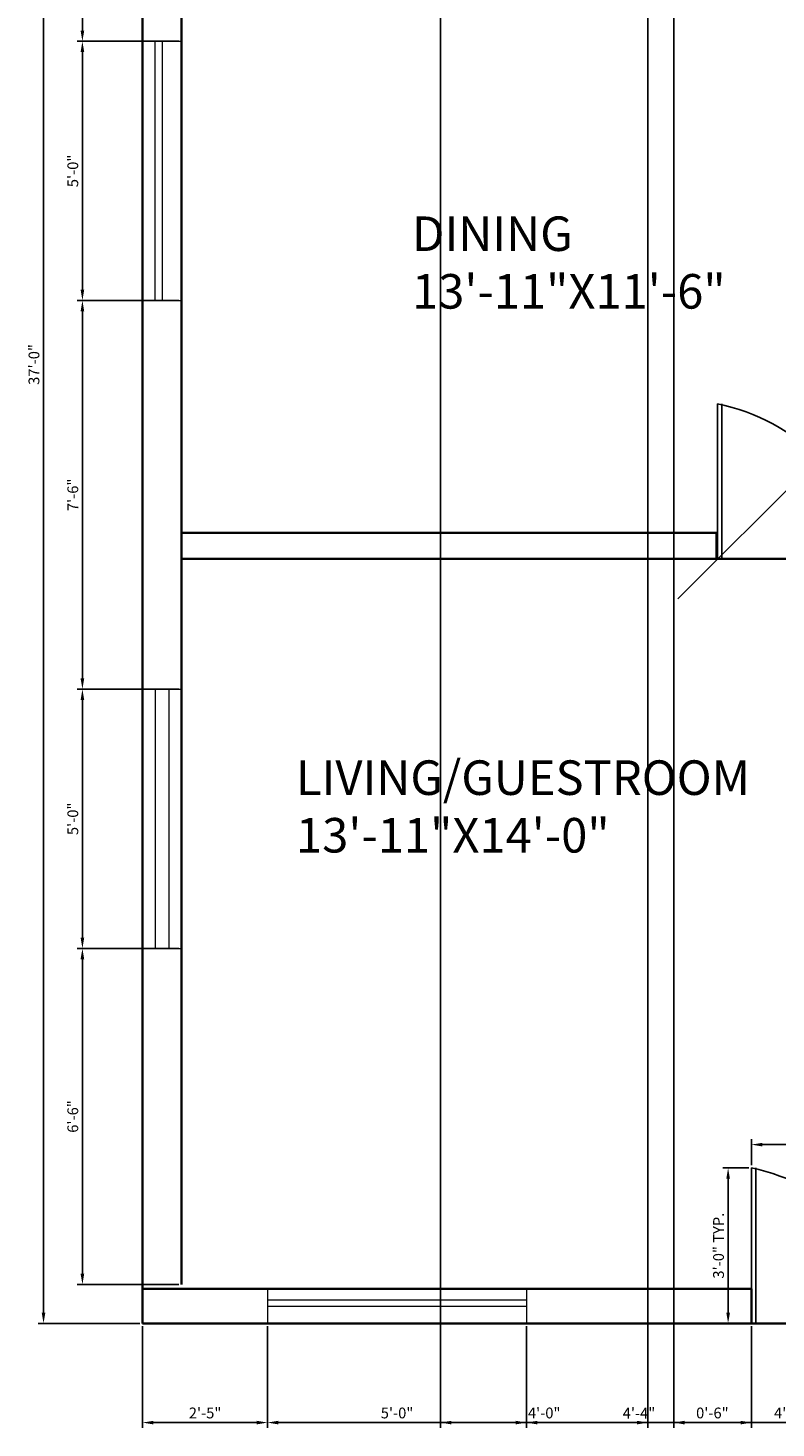
# Model space of a CAD drawing. Units: inches. Extents: x -2945 to -2182, y 3541 to 4172.
# Tile 3 of 5: x -2558 to -2384, y 3541 to 3865. Entities that reach past the tile are written whole.
import ezdxf

# ---------------------------------------------------------------- set-up
doc = ezdxf.new("R2010")
doc.units = ezdxf.units.IN
for name, color, linetype, lineweight in [('A-ANNO-DIMS', 2, 'Continuous', 18), ('A-AREA-IDEN', 7, 'Continuous', 18), ('A-DOOR', 3, 'Continuous', 25), ('A-GLAZ', 4, 'Continuous', 18), ('A-WALL', 7, 'Continuous', 35)]:
    doc.layers.add(name, color=color, linetype=linetype, lineweight=lineweight)
doc.styles.get("Standard").update_dxf_attribs({"font": 'arial.ttf'})
doc.dimstyles.new('ISO-25', dxfattribs={"dimtxt": 2.5, "dimasz": 2.5, "dimexe": 1.25, "dimexo": 0.625, "dimtad": 1, "dimdec": 0, "dimlunit": 3, "dimtxsty": 'Standard', "dimcen": 2.5, "dimadec": 0, "dimazin": 0, "dimtfac": 1, "dimtdec": 0, "dimtmove": 0, "dimatfit": 3, "dimfxl": 1, "dimarcsym": 0})

# ---------------------------------------------------------------- blocks, each defined once
blk = doc.blocks.new('DOOR-SINGLE-36IN')
for p, q in [((0, 0), (0, 36)), ((1, 0), (1, 36))]:
    blk.add_line(p, q)
blk.add_arc((-9.18, -9.18), 46.1, 11.4852, 78.5148)
blk = doc.blocks.new('*D18')
at = {"layer": 'A-ANNO-DIMS', "color": 0, "lineweight": -2, "transparency": 16777216}
for p, q in [((-2390.05, 3602.2), (-2390.05, 3608.23)), ((-2354.05, 3602.2), (-2354.05, 3608.23)), ((-2387.55, 3606.98), (-2356.55, 3606.98)), ((-2354.05, 3606.98), (-2309.84, 3606.98))]:
    blk.add_line(p, q, dxfattribs=at)
at = {"layer": 'A-ANNO-DIMS', "color": 0, "transparency": 16777216}
for points in [[(-2387.55, 3607.39), (-2387.55, 3606.56), (-2390.05, 3606.98)], [(-2356.55, 3607.39), (-2356.55, 3606.56), (-2354.05, 3606.98)]]:
    blk.add_solid(points, dxfattribs=at)
at = {"layer": 'Defpoints', "color": 0, "transparency": 16777216}
for p in [(-2354.05, 3606.98), (-2390.05, 3601.58), (-2354.05, 3601.58)]:
    blk.add_point(p, dxfattribs=at)
at = {"layer": 'A-ANNO-DIMS', "color": 0, "transparency": 16777216, "insert": (-2330.7, 3608.89), "char_height": 2.5, "attachment_point": 5}
blk.add_mtext('SINGLE DOOR 3\'-0" TYP.', dxfattribs=at)
blk = doc.blocks.new('*D19')
at = {"layer": 'A-ANNO-DIMS', "color": 0, "lineweight": -2, "transparency": 16777216}
for p, q in [((-2390.67, 3601.58), (-2396.7, 3601.58)), ((-2395.45, 3568.08), (-2395.45, 3599.08)), ((-2390.67, 3565.58), (-2396.7, 3565.58))]:
    blk.add_line(p, q, dxfattribs=at)
at = {"layer": 'A-ANNO-DIMS', "color": 0, "transparency": 16777216}
for points in [[(-2395.87, 3599.08), (-2395.03, 3599.08), (-2395.45, 3601.58)], [(-2395.87, 3568.08), (-2395.03, 3568.08), (-2395.45, 3565.58)]]:
    blk.add_solid(points, dxfattribs=at)
at = {"layer": 'Defpoints', "color": 0, "transparency": 16777216}
for p in [(-2395.45, 3601.58), (-2390.05, 3601.58), (-2390.05, 3565.58)]:
    blk.add_point(p, dxfattribs=at)
at = {"layer": 'A-ANNO-DIMS', "color": 0, "transparency": 16777216, "insert": (-2397.35, 3583.58), "char_height": 2.5, "attachment_point": 5, "rotation": 90}
blk.add_mtext('3\'-0" TYP.', dxfattribs=at)
blk = doc.blocks.new('*D21')
at = {"layer": 'A-ANNO-DIMS', "color": 0, "lineweight": -2, "transparency": 16777216}
for p, q in [((-2531.67, 4009.58), (-2555.25, 4009.58)), ((-2554, 3568.08), (-2554, 4007.08)), ((-2531.67, 3565.58), (-2555.25, 3565.58))]:
    blk.add_line(p, q, dxfattribs=at)
at = {"layer": 'A-ANNO-DIMS', "color": 0, "transparency": 16777216}
for points in [[(-2554.42, 4007.08), (-2553.58, 4007.08), (-2554, 4009.58)], [(-2554.42, 3568.08), (-2553.58, 3568.08), (-2554, 3565.58)]]:
    blk.add_solid(points, dxfattribs=at)
at = {"layer": 'Defpoints', "color": 0, "transparency": 16777216}
for p in [(-2554, 4009.58), (-2531.05, 4009.58), (-2531.05, 3565.58)]:
    blk.add_point(p, dxfattribs=at)
at = {"layer": 'A-ANNO-DIMS', "color": 0, "transparency": 16777216, "insert": (-2555.9, 3787.58), "char_height": 2.5, "attachment_point": 5, "rotation": 90}
blk.add_mtext('37\'-0"', dxfattribs=at)
blk = doc.blocks.new('*D22')
at = {"layer": 'A-ANNO-DIMS', "color": 0, "lineweight": -2, "transparency": 16777216}
for p, q in [((-2531.05, 3564.95), (-2531.05, 3541.38)), ((-2502.13, 3564.95), (-2502.13, 3541.38)), ((-2528.55, 3542.63), (-2504.63, 3542.63))]:
    blk.add_line(p, q, dxfattribs=at)
at = {"layer": 'A-ANNO-DIMS', "color": 0, "transparency": 16777216}
for points in [[(-2528.55, 3543.04), (-2528.55, 3542.21), (-2531.05, 3542.63)], [(-2504.63, 3543.04), (-2504.63, 3542.21), (-2502.13, 3542.63)]]:
    blk.add_solid(points, dxfattribs=at)
at = {"layer": 'Defpoints', "color": 0, "transparency": 16777216}
for p in [(-2531.05, 3565.58), (-2502.13, 3565.58), (-2502.13, 3542.63)]:
    blk.add_point(p, dxfattribs=at)
at = {"layer": 'A-ANNO-DIMS', "color": 0, "transparency": 16777216, "insert": (-2516.59, 3544.53), "char_height": 2.5, "attachment_point": 5}
blk.add_mtext('2\'-5"', dxfattribs=at)
blk = doc.blocks.new('*D23')
at = {"layer": 'A-ANNO-DIMS', "color": 0, "lineweight": -2, "transparency": 16777216}
for p, q in [((-2502.13, 3564.95), (-2502.13, 3541.38)), ((-2442.13, 3564.95), (-2442.13, 3541.38)), ((-2499.63, 3542.63), (-2444.63, 3542.63))]:
    blk.add_line(p, q, dxfattribs=at)
at = {"layer": 'A-ANNO-DIMS', "color": 0, "transparency": 16777216}
for points in [[(-2499.63, 3543.04), (-2499.63, 3542.21), (-2502.13, 3542.63)], [(-2444.63, 3543.04), (-2444.63, 3542.21), (-2442.13, 3542.63)]]:
    blk.add_solid(points, dxfattribs=at)
at = {"layer": 'Defpoints', "color": 0, "transparency": 16777216}
for p in [(-2502.13, 3565.58), (-2442.13, 3565.58), (-2442.13, 3542.63)]:
    blk.add_point(p, dxfattribs=at)
at = {"layer": 'A-ANNO-DIMS', "color": 0, "transparency": 16777216, "insert": (-2472.13, 3544.53), "char_height": 2.5, "attachment_point": 5}
blk.add_mtext('5\'-0"', dxfattribs=at)
blk = doc.blocks.new('*D24')
at = {"layer": 'A-ANNO-DIMS', "color": 0, "lineweight": -2, "transparency": 16777216}
for p, q in [((-2442.13, 3564.95), (-2442.13, 3541.38)), ((-2390.05, 3564.95), (-2390.05, 3541.38)), ((-2439.63, 3542.63), (-2392.55, 3542.63))]:
    blk.add_line(p, q, dxfattribs=at)
at = {"layer": 'A-ANNO-DIMS', "color": 0, "transparency": 16777216}
for points in [[(-2439.63, 3543.04), (-2439.63, 3542.21), (-2442.13, 3542.63)], [(-2392.55, 3543.04), (-2392.55, 3542.21), (-2390.05, 3542.63)]]:
    blk.add_solid(points, dxfattribs=at)
at = {"layer": 'Defpoints', "color": 0, "transparency": 16777216}
for p in [(-2442.13, 3565.58), (-2390.05, 3565.58), (-2390.05, 3542.63)]:
    blk.add_point(p, dxfattribs=at)
at = {"layer": 'A-ANNO-DIMS', "color": 0, "transparency": 16777216, "insert": (-2416.09, 3544.5), "char_height": 2.5, "attachment_point": 5}
blk.add_mtext('4\'-4"', dxfattribs=at)
blk = doc.blocks.new('*D25')
at = {"layer": 'A-ANNO-DIMS', "color": 0, "lineweight": -2, "transparency": 16777216}
for p, q in [((-2522.67, 3652.4), (-2546.25, 3652.4)), ((-2545, 3577.08), (-2545, 3649.9)), ((-2522.67, 3574.58), (-2546.25, 3574.58))]:
    blk.add_line(p, q, dxfattribs=at)
at = {"layer": 'A-ANNO-DIMS', "color": 0, "transparency": 16777216}
for points in [[(-2545.42, 3649.9), (-2544.58, 3649.9), (-2545, 3652.4)], [(-2545.42, 3577.08), (-2544.58, 3577.08), (-2545, 3574.58)]]:
    blk.add_solid(points, dxfattribs=at)
at = {"layer": 'Defpoints', "color": 0, "transparency": 16777216}
for p in [(-2545, 3652.4), (-2522.05, 3652.4), (-2522.05, 3574.58)]:
    blk.add_point(p, dxfattribs=at)
at = {"layer": 'A-ANNO-DIMS', "color": 0, "transparency": 16777216, "insert": (-2546.9, 3613.49), "char_height": 2.5, "attachment_point": 5, "rotation": 90}
blk.add_mtext('6\'-6"', dxfattribs=at)
blk = doc.blocks.new('*D26')
at = {"layer": 'A-ANNO-DIMS', "color": 0, "lineweight": -2, "transparency": 16777216}
for p, q in [((-2522.67, 3712.4), (-2546.25, 3712.4)), ((-2545, 3654.9), (-2545, 3709.9)), ((-2522.67, 3652.4), (-2546.25, 3652.4))]:
    blk.add_line(p, q, dxfattribs=at)
at = {"layer": 'A-ANNO-DIMS', "color": 0, "transparency": 16777216}
for points in [[(-2545.42, 3709.9), (-2544.58, 3709.9), (-2545, 3712.4)], [(-2545.42, 3654.9), (-2544.58, 3654.9), (-2545, 3652.4)]]:
    blk.add_solid(points, dxfattribs=at)
at = {"layer": 'Defpoints', "color": 0, "transparency": 16777216}
for p in [(-2545, 3712.4), (-2522.05, 3712.4), (-2522.05, 3652.4)]:
    blk.add_point(p, dxfattribs=at)
at = {"layer": 'A-ANNO-DIMS', "color": 0, "transparency": 16777216, "insert": (-2546.9, 3682.4), "char_height": 2.5, "attachment_point": 5, "rotation": 90}
blk.add_mtext('5\'-0"', dxfattribs=at)
blk = doc.blocks.new('*D27')
at = {"layer": 'A-ANNO-DIMS', "color": 0, "lineweight": -2, "transparency": 16777216}
for p, q in [((-2522.67, 3802.39), (-2546.25, 3802.39)), ((-2545, 3714.9), (-2545, 3799.89)), ((-2522.67, 3712.4), (-2546.25, 3712.4))]:
    blk.add_line(p, q, dxfattribs=at)
at = {"layer": 'A-ANNO-DIMS', "color": 0, "transparency": 16777216}
for points in [[(-2545.42, 3799.89), (-2544.58, 3799.89), (-2545, 3802.39)], [(-2545.42, 3714.9), (-2544.58, 3714.9), (-2545, 3712.4)]]:
    blk.add_solid(points, dxfattribs=at)
at = {"layer": 'Defpoints', "color": 0, "transparency": 16777216}
for p in [(-2545, 3802.39), (-2522.05, 3802.39), (-2522.05, 3712.4)]:
    blk.add_point(p, dxfattribs=at)
at = {"layer": 'A-ANNO-DIMS', "color": 0, "transparency": 16777216, "insert": (-2546.9, 3757.4), "char_height": 2.5, "attachment_point": 5, "rotation": 90}
blk.add_mtext('7\'-6"', dxfattribs=at)
blk = doc.blocks.new('*D28')
at = {"layer": 'A-ANNO-DIMS', "color": 0, "lineweight": -2, "transparency": 16777216}
for p, q in [((-2522.67, 3862.39), (-2546.25, 3862.39)), ((-2545, 3804.89), (-2545, 3859.89)), ((-2522.67, 3802.39), (-2546.25, 3802.39))]:
    blk.add_line(p, q, dxfattribs=at)
at = {"layer": 'A-ANNO-DIMS', "color": 0, "transparency": 16777216}
for points in [[(-2545.42, 3859.89), (-2544.58, 3859.89), (-2545, 3862.39)], [(-2545.42, 3804.89), (-2544.58, 3804.89), (-2545, 3802.39)]]:
    blk.add_solid(points, dxfattribs=at)
at = {"layer": 'Defpoints', "color": 0, "transparency": 16777216}
for p in [(-2545, 3862.39), (-2522.05, 3862.39), (-2522.05, 3802.39)]:
    blk.add_point(p, dxfattribs=at)
at = {"layer": 'A-ANNO-DIMS', "color": 0, "transparency": 16777216, "insert": (-2546.9, 3832.39), "char_height": 2.5, "attachment_point": 5, "rotation": 90}
blk.add_mtext('5\'-0"', dxfattribs=at)
blk = doc.blocks.new('*D29')
at = {"layer": 'A-ANNO-DIMS', "color": 0, "lineweight": -2, "transparency": 16777216}
for p, q in [((-2522.67, 3935.75), (-2546.25, 3935.75)), ((-2545, 3864.89), (-2545, 3933.25)), ((-2522.67, 3862.39), (-2546.25, 3862.39))]:
    blk.add_line(p, q, dxfattribs=at)
at = {"layer": 'A-ANNO-DIMS', "color": 0, "transparency": 16777216}
for points in [[(-2545.42, 3933.25), (-2544.58, 3933.25), (-2545, 3935.75)], [(-2545.42, 3864.89), (-2544.58, 3864.89), (-2545, 3862.39)]]:
    blk.add_solid(points, dxfattribs=at)
at = {"layer": 'Defpoints', "color": 0, "transparency": 16777216}
for p in [(-2545, 3935.75), (-2522.05, 3935.75), (-2522.05, 3862.39)]:
    blk.add_point(p, dxfattribs=at)
at = {"layer": 'A-ANNO-DIMS', "color": 0, "transparency": 16777216, "insert": (-2546.92, 3899.07), "char_height": 2.5, "attachment_point": 5, "rotation": 90}
blk.add_mtext('6\'-1 1/2"', dxfattribs=at)
blk = doc.blocks.new('*D41')
at = {"layer": 'A-ANNO-DIMS', "color": 0, "lineweight": -2, "transparency": 16777216}
for p, q in [((-2408.05, 3920.95), (-2408.05, 3541.38)), ((-2354.05, 3920.95), (-2354.05, 3541.38)), ((-2405.55, 3542.63), (-2356.55, 3542.63))]:
    blk.add_line(p, q, dxfattribs=at)
at = {"layer": 'A-ANNO-DIMS', "color": 0, "transparency": 16777216}
for points in [[(-2405.55, 3543.04), (-2405.55, 3542.21), (-2408.05, 3542.63)], [(-2356.55, 3543.04), (-2356.55, 3542.21), (-2354.05, 3542.63)]]:
    blk.add_solid(points, dxfattribs=at)
at = {"layer": 'Defpoints', "color": 0, "transparency": 16777216}
for p in [(-2408.05, 3921.58), (-2354.05, 3921.58), (-2354.05, 3542.63)]:
    blk.add_point(p, dxfattribs=at)
at = {"layer": 'A-ANNO-DIMS', "color": 0, "transparency": 16777216, "insert": (-2381.05, 3544.53), "char_height": 2.5, "attachment_point": 5}
blk.add_mtext('4\'-6"', dxfattribs=at)
blk = doc.blocks.new('*D45')
at = {"layer": 'A-ANNO-DIMS', "color": 0, "lineweight": -2, "transparency": 16777216}
for p, q in [((-2414.05, 3885.95), (-2414.05, 3541.38)), ((-2408.05, 3885.95), (-2408.05, 3541.38)), ((-2416.55, 3542.63), (-2419.05, 3542.63)), ((-2414.05, 3542.63), (-2408.05, 3542.63)), ((-2405.55, 3542.63), (-2395.15, 3542.63))]:
    blk.add_line(p, q, dxfattribs=at)
at = {"layer": 'A-ANNO-DIMS', "color": 0, "transparency": 16777216}
for points in [[(-2416.55, 3543.04), (-2416.55, 3542.21), (-2414.05, 3542.63)], [(-2405.55, 3543.04), (-2405.55, 3542.21), (-2408.05, 3542.63)]]:
    blk.add_solid(points, dxfattribs=at)
at = {"layer": 'Defpoints', "color": 0, "transparency": 16777216}
for p in [(-2414.05, 3886.58), (-2408.05, 3886.58), (-2408.05, 3542.63)]:
    blk.add_point(p, dxfattribs=at)
at = {"layer": 'A-ANNO-DIMS', "color": 0, "transparency": 16777216, "insert": (-2399.1, 3544.53), "char_height": 2.5, "attachment_point": 5}
blk.add_mtext('0\'-6"', dxfattribs=at)
blk = doc.blocks.new('*D47')
at = {"layer": 'A-ANNO-DIMS', "color": 0, "lineweight": -2, "transparency": 16777216}
for p, q in [((-2462.05, 3885.95), (-2462.05, 3541.38)), ((-2414.05, 3885.95), (-2414.05, 3541.38)), ((-2459.55, 3542.63), (-2416.55, 3542.63))]:
    blk.add_line(p, q, dxfattribs=at)
at = {"layer": 'A-ANNO-DIMS', "color": 0, "transparency": 16777216}
for points in [[(-2459.55, 3543.04), (-2459.55, 3542.21), (-2462.05, 3542.63)], [(-2416.55, 3543.04), (-2416.55, 3542.21), (-2414.05, 3542.63)]]:
    blk.add_solid(points, dxfattribs=at)
at = {"layer": 'Defpoints', "color": 0, "transparency": 16777216}
for p in [(-2462.05, 3886.58), (-2414.05, 3886.58), (-2414.05, 3542.63)]:
    blk.add_point(p, dxfattribs=at)
at = {"layer": 'A-ANNO-DIMS', "color": 0, "transparency": 16777216, "insert": (-2438.05, 3544.53), "char_height": 2.5, "attachment_point": 5}
blk.add_mtext('4\'-0"', dxfattribs=at)
blk = doc.blocks.new('*D77')
at = {"layer": 'A-ANNO-DIMS', "color": 0, "lineweight": -2, "transparency": 16777216}
for p, q in [((-2350.58, 3789.78), (-2372.69, 3767.66)), ((-2407.06, 3733.29), (-2374.46, 3765.89))]:
    blk.add_line(p, q, dxfattribs=at)
at = {"layer": 'A-ANNO-DIMS', "color": 0, "transparency": 16777216}
blk.add_solid([(-2372.99, 3767.96), (-2372.4, 3767.37), (-2374.46, 3765.89)], dxfattribs=at)
at = {"layer": 'Defpoints', "color": 0, "transparency": 16777216}
for p in [(-2374.46, 3765.89), (-2407.06, 3733.29)]:
    blk.add_point(p, dxfattribs=at)
at = {"layer": 'A-ANNO-DIMS', "color": 0, "transparency": 16777216, "insert": (-2356.24, 3786.8), "char_height": 2.5, "attachment_point": 5, "rotation": 44.9998}
blk.add_mtext('R3\'-10"', dxfattribs=at)

msp = doc.modelspace()

# ---------------------------------------------------------------- linework, layer by layer
at = {"layer": 'A-GLAZ'}
for p, q in [((-2531.05, 3862.39), (-2522.05, 3862.39)), ((-2528.26, 3862.39), (-2528.26, 3802.39)), ((-2526.55, 3862.39), (-2526.55, 3802.39)), ((-2531.05, 3802.39), (-2522.05, 3802.39)), ((-2531.05, 3712.4), (-2522.05, 3712.4)), ((-2528.11, 3652.4), (-2528.11, 3712.4)), ((-2524.96, 3712.4), (-2524.96, 3652.4)), ((-2531.05, 3652.4), (-2522.05, 3652.4)), ((-2502.13, 3573.58), (-2502.13, 3565.58)), ((-2442.13, 3573.58), (-2442.13, 3565.58)), ((-2502.13, 3571.08), (-2442.13, 3571.08)), ((-2502.13, 3569.58), (-2442.13, 3569.58))]:
    msp.add_line(p, q, dxfattribs=at)
at = {"layer": 'A-WALL'}
for p, q in [((-2531.05, 3565.58), (-2531.05, 4009.58)), ((-2522.05, 3574.58), (-2522.05, 4000.58)), ((-2522.05, 3748.58), (-2398.11, 3748.58)), ((-2398.11, 3748.58), (-2398.11, 3742.58)), ((-2522.05, 3742.58), (-2354.05, 3742.58)), ((-2390.05, 3573.58), (-2531.05, 3573.58)), ((-2390.05, 3573.58), (-2390.05, 3565.58)), ((-2207.05, 3565.58), (-2531.05, 3565.58))]:
    msp.add_line(p, q, dxfattribs=at)

# ---------------------------------------------------------------- block references
at = {"layer": 'A-DOOR'}
for p in [(-2397.88, 3742.47), (-2390.05, 3565.57)]:
    msp.add_blockref('DOOR-SINGLE-36IN', p, dxfattribs=at)

# ---------------------------------------------------------------- texts
at = {"layer": 'A-AREA-IDEN', "char_height": 8, "attachment_point": 1}
for s, width, heights, insert in [('DINING\\P13\'-11"X11\'-6"', 51.4369, [29.22], (-2468.66, 3821.85)), ('LIVING/GUESTROOM\\P13\'-11"X14\'-0"', 104.8493, [0], (-2495.53, 3695.93))]:
    msp.add_mtext_dynamic_manual_height_columns(s, width=width, gutter_width=12.5, heights=heights, dxfattribs=dict(at, insert=insert))

# ---------------------------------------------------------------- dimensions: what is measured, and where the dimension line sits
at = {"layer": 'A-ANNO-DIMS'}
for base, p1, p2, picture, middle in [((-2554, 4009.58), (-2531.05, 3565.58), (-2531.05, 4009.58), '*D21', (-2555.9, 3787.58)), ((-2545, 3935.75), (-2522.05, 3862.39), (-2522.05, 3935.75), '*D29', (-2546.92, 3899.07)), ((-2545, 3862.39), (-2522.05, 3802.39), (-2522.05, 3862.39), '*D28', (-2546.9, 3832.39)), ((-2545, 3802.39), (-2522.05, 3712.4), (-2522.05, 3802.39), '*D27', (-2546.9, 3757.4)), ((-2545, 3712.4), (-2522.05, 3652.4), (-2522.05, 3712.4), '*D26', (-2546.9, 3682.4)), ((-2545, 3652.4), (-2522.05, 3574.58), (-2522.05, 3652.4), '*D25', (-2546.9, 3613.49))]:
    dim = msp.add_linear_dim(base=base, p1=p1, p2=p2, angle=90, dimstyle='ISO-25', override={"dimdec": 1, "dimlfac": 1, "dimrnd": 0, "dimzin": 1, "dimdsep": 46, "dimlunit": 4, "dimfrac": 2}, dxfattribs=at)
    dim.commit()
    dim.dimension.update_dxf_attribs({"geometry": picture, "text_midpoint": middle})
for base, p1, p2, picture, middle in [((-2354.05, 3542.63), (-2408.05, 3921.58), (-2354.05, 3921.58), '*D41', (-2381.05, 3544.53)), ((-2414.05, 3542.63), (-2462.05, 3886.58), (-2414.05, 3886.58), '*D47', (-2438.05, 3544.53)), ((-2408.05, 3542.63), (-2414.05, 3886.58), (-2408.05, 3886.58), '*D45', (-2399.1, 3544.53)), ((-2502.13, 3542.63), (-2531.05, 3565.58), (-2502.13, 3565.58), '*D22', (-2516.59, 3544.53)), ((-2442.13, 3542.63), (-2502.13, 3565.58), (-2442.13, 3565.58), '*D23', (-2472.13, 3544.53)), ((-2390.05, 3542.63), (-2442.13, 3565.58), (-2390.05, 3565.58), '*D24', (-2416.09, 3544.5))]:
    dim = msp.add_linear_dim(base=base, p1=p1, p2=p2, dimstyle='ISO-25', override={"dimdec": 1, "dimlfac": 1, "dimrnd": 0, "dimzin": 1, "dimdsep": 46, "dimlunit": 4, "dimfrac": 2}, dxfattribs=at)
    dim.commit()
    dim.dimension.update_dxf_attribs({"geometry": picture, "text_midpoint": middle})
dim = msp.add_radius_dim(center=(-2407.06, 3733.29), mpoint=(-2374.46, 3765.89), dimstyle='ISO-25', override={"dimdec": 1, "dimlfac": 1, "dimrnd": 0, "dimzin": 1, "dimdsep": 46, "dimlunit": 4, "dimfrac": 2}, dxfattribs=at)
dim.commit()
dim.dimension.update_dxf_attribs({"geometry": '*D77', "text_midpoint": (-2354.9, 3785.45), "dimtype": 164})
dim = msp.add_linear_dim(base=(-2354.05, 3606.98), p1=(-2390.05, 3601.58), p2=(-2354.05, 3601.58), text='SINGLE DOOR <> TYP.', dimstyle='ISO-25', override={"dimdec": 1, "dimlfac": 1, "dimrnd": 0, "dimzin": 1, "dimdsep": 46, "dimlunit": 4, "dimfrac": 2}, dxfattribs=at)
dim.commit()
dim.dimension.update_dxf_attribs({"geometry": '*D18', "text_midpoint": (-2330.7, 3608.89)})
dim = msp.add_linear_dim(base=(-2395.45, 3601.58), p1=(-2390.05, 3565.58), p2=(-2390.05, 3601.58), angle=90, text='<> TYP.', dimstyle='ISO-25', override={"dimdec": 1, "dimlfac": 1, "dimrnd": 0, "dimzin": 1, "dimdsep": 46, "dimlunit": 4, "dimfrac": 2}, dxfattribs=at)
dim.commit()
dim.dimension.update_dxf_attribs({"geometry": '*D19', "text_midpoint": (-2397.35, 3583.58)})

doc.saveas('drawing.dxf')
